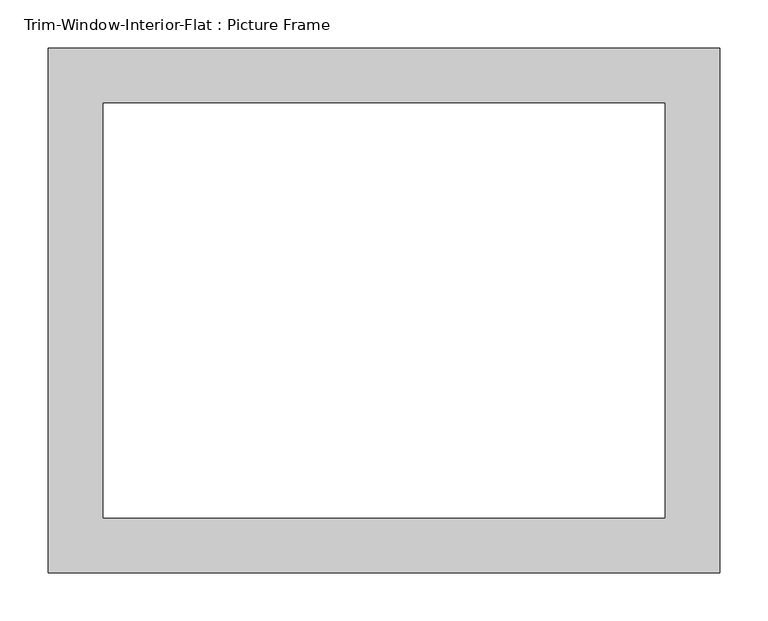
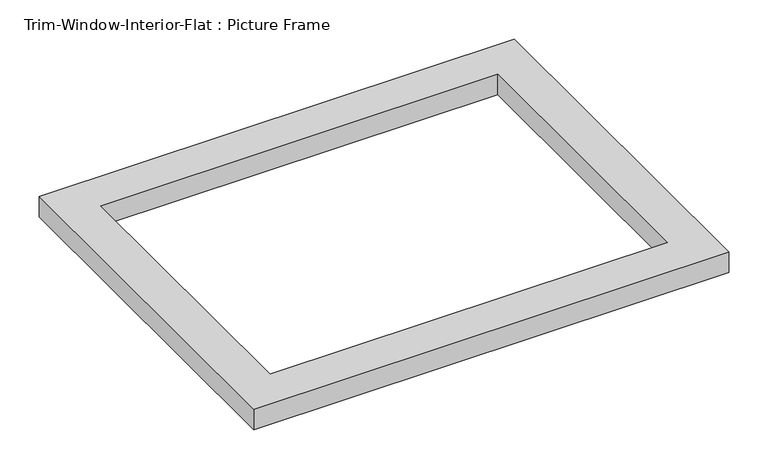
"""IFC4 building model written with IfcOpenShell, lengths in millimetres: proxy geometry, Trim-Window-Interior-Flat : Picture Frame."""

from ifc_helpers import new_model, si_unit, origin, origin_with_axes, place, context, project, spatial, polyline, outline, extrude, source, transform, mapped, element, save


def trim_window_interior_flat_picture_frame_f985c0ae(model_context):
    return source(origin(), model_context, "Body", "SweptSolid", [
        extrude(outline(polyline([(349.25, 44.45), (349.25, -501.65), (-349.25, -501.65), (-349.25, 44.45), (349.25, 44.45)]), holes=[polyline([(292.1, -12.7), (-292.1, -12.7), (-292.1, -444.5), (292.1, -444.5), (292.1, -12.7)])]), origin_with_axes(), (0.0, 0.0, 1.0), 31.75),
    ])


if __name__ == "__main__":
    model = new_model("IFC4")
    model_context = context("Model", 3, world=origin())
    ifc_project = project(units=[si_unit("LENGTHUNIT", "METRE", prefix="MILLI")], contexts=[model_context])
    site = spatial("IfcSite", under=ifc_project)
    building = spatial("IfcBuilding", under=site)
    placement = place(None, origin())
    trim_window_interior_flat_picture_frame_shape = trim_window_interior_flat_picture_frame_f985c0ae(model_context)
    element("IfcBuildingElementProxy", 1, Name="Trim-Window-Interior-Flat : Picture Frame", ObjectType="Trim-Window-Interior-Flat : Picture Frame", at=placement, inside=building, context=model_context, shape_type="MappedRepresentation", body=[
        mapped(trim_window_interior_flat_picture_frame_shape, transform((0.0, 0.0, 0.0), x_axis=(1.0, 0.0, 0.0), y_axis=(0.0, 1.0, 0.0), z_axis=(0.0, 0.0, 1.0))),
    ])
    save(model, "model.ifc")

# Revit data of these elements
# Type "Trim-Window-Interior-Flat : Picture Frame"
#   Trim Thickness_Picture Frame = 0' - 1 1/4"
#   Trim Width = 0' - 2 1/4"
#   Trim Thickness_with Sill = 0' - 0 3/4"
#   Sill Thickness = 0' - 1 1/4"
#   Opening Width [instance default] = 2' - 0"
#   Opening Height [instance default] = 3' - 0"
#   Default Elevation = 4' - 0"
#   Sill = no
#   Picture Frame = yes
#   Trim Material [instance default] = none
# Element 1 (IfcBuildingElementProxy, "Trim-Window-Interior-Flat : Picture Frame")
#   Opening Height = 1' - 6"
#   Trim Material = Wood - Stained
#   Materials on its faces: "Wood - Stained"
# Materials
#   "Wood - Stained": class "Wood", colour RGB 224 178 126, transparency 0, Cost = 0
